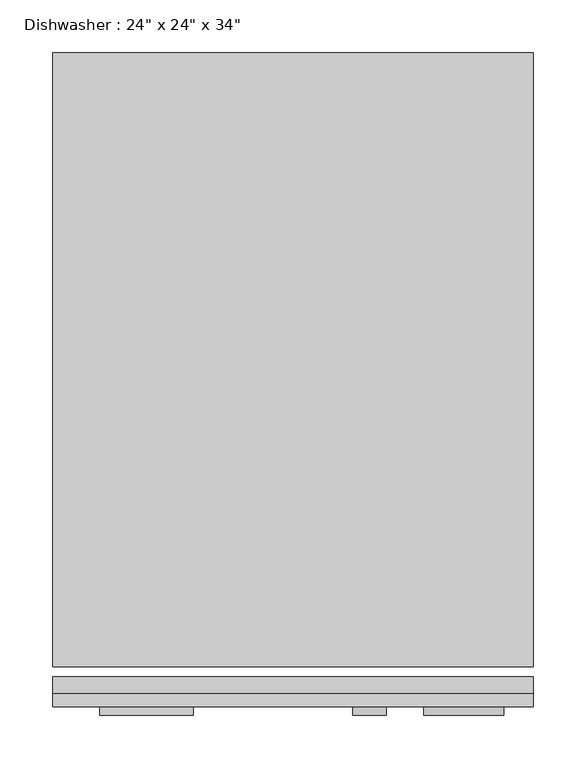
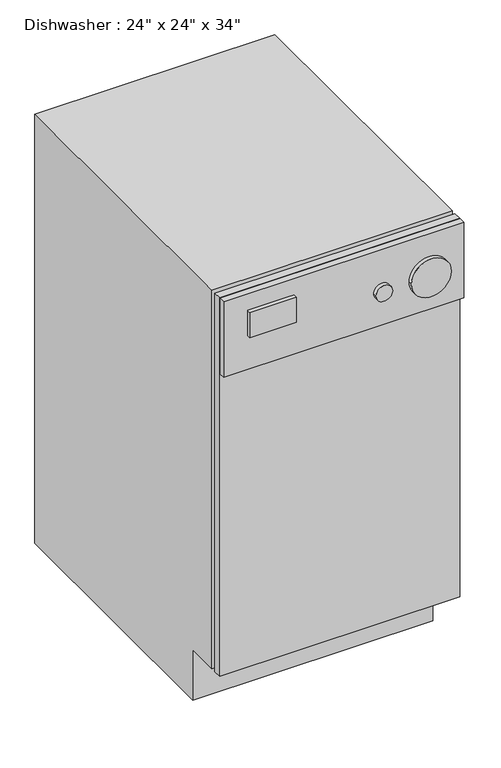
"""IFC4 building model written with IfcOpenShell, lengths in millimetres: proxy geometry."""

from ifc_helpers import new_model, si_unit, point, frame, frame_2d, origin, place, context, project, spatial, polyline, circle_curve, trimmed, segment, composite_curve, outline, extrude, source, transform, mapped, element, save


def proxy_434a9211(model_context):
    return source(origin(), model_context, "Body", "SweptSolid", [
        extrude(outline(polyline([(534.7174685, -38.3504352), (77.5174685, -38.3504352), (77.5174685, -22.4754352), (534.7174685, -22.4754352), (534.7174685, -38.3504352)])), frame((0.0, 0.0, 101.6), z_axis=(0.0, 0.0, 1.0), x_axis=(1.0, 0.0, 0.0)), (0.0, 0.0, 1.0), 762.0),
        extrude(outline(polyline([(534.7174685, -38.3504352), (534.7174685, -51.0504352), (77.5174685, -51.0504352), (77.5174685, -38.3504352), (534.7174685, -38.3504352)])), frame((0.0, 0.0, 711.2), z_axis=(0.0, 0.0, 1.0), x_axis=(1.0, 0.0, 0.0)), (0.0, 0.0, 1.0), 152.4),
        extrude(outline(polyline([(571.2495648, 0.0), (50.5495648, 0.0), (50.5495648, 101.6), (-12.9504352, 101.6), (-12.9504352, 863.6), (571.2495648, 863.6), (571.2495648, 0.0)])), frame((77.5174685, 0.0, 0.0), z_axis=(1.0, 0.0, 0.0), x_axis=(0.0, 1.0, 0.0)), (0.0, 0.0, 1.0), 457.2),
        extrude(outline(polyline([(211.4378068, -59.1863727), (122.5378068, -59.1863727), (122.5378068, -51.0504352), (211.4378068, -51.0504352), (211.4378068, -59.1863727)])), frame((0.0, 0.0, 780.0846419), z_axis=(0.0, 0.0, 1.0), x_axis=(1.0, 0.0, 0.0)), (0.0, 0.0, 1.0), 50.8),
        extrude(outline(composite_curve([segment(trimmed(circle_curve(frame_2d((780.0846419, 468.5247133)), 38.1), [point((780.0846419, 430.4247133))], [point((780.0846419, 506.6247133))], False, "CARTESIAN"), True, "CONTINUOUS"), segment(trimmed(circle_curve(frame_2d((780.0846419, 468.5247133)), 38.1), [point((780.0846419, 506.6247133))], [point((780.0846419, 430.4247133))], False, "CARTESIAN"), True, "CONTINUOUS")], self_intersect=False)), frame((0.0, -59.1863727, 0.0), z_axis=(0.0, 1.0, 0.0), x_axis=(0.0, 0.0, 1.0)), (0.0, 0.0, 1.0), 8.1359375),
        extrude(outline(composite_curve([segment(trimmed(circle_curve(frame_2d((780.0846419, 378.995318)), 15.875), [point((780.0846419, 363.120318))], [point((780.0846419, 394.870318))], False, "CARTESIAN"), True, "CONTINUOUS"), segment(trimmed(circle_curve(frame_2d((780.0846419, 378.995318)), 15.875), [point((780.0846419, 394.870318))], [point((780.0846419, 363.120318))], False, "CARTESIAN"), True, "CONTINUOUS")], self_intersect=False)), frame((0.0, -59.1863727, 0.0), z_axis=(0.0, 1.0, 0.0), x_axis=(0.0, 0.0, 1.0)), (0.0, 0.0, 1.0), 8.1359375),
    ])


if __name__ == "__main__":
    model = new_model("IFC4")
    model_context = context("Model", 3, world=origin())
    ifc_project = project(units=[si_unit("LENGTHUNIT", "METRE", prefix="MILLI")], contexts=[model_context])
    site = spatial("IfcSite", under=ifc_project)
    building = spatial("IfcBuilding", under=site)
    placement = place(None, origin())
    proxy_shape = proxy_434a9211(model_context)
    element("IfcBuildingElementProxy", 1, Name="Dishwasher : 24\" x 24\" x 34\"", ObjectType="Dishwasher : 24\" x 24\" x 34\"", at=placement, inside=building, context=model_context, shape_type="MappedRepresentation", body=[
        mapped(proxy_shape, transform((0.0, 0.0, 0.0), x_axis=(1.0, 0.0, 0.0), y_axis=(0.0, 1.0, 0.0), z_axis=(0.0, 0.0, 1.0))),
    ])
    save(model, "model.ifc")

# Revit data of these elements
# Type "Dishwasher : 24\" x 24\" x 34\""
#   Label = "DW"
#   Assembly Code = "E1090400"
#   Depth = 2' - 0"
#   Height = 2' - 10"
#   Width = 1' - 6"
#   Dishwasher Material = Steel, Paint Finish, Ivory, Glossy
#   Panel Face Material = Plastic, Opaque Black
#   Default Elevation = 0
# Element 1 (IfcBuildingElementProxy, "Dishwasher : 24\" x 24\" x 34\"")
#   Materials on its faces: "Steel, Paint Finish, Ivory, Glossy", "Plastic, Opaque Black"
# Materials
#   "Steel, Paint Finish, Ivory, Glossy": class "Metal", colour RGB 247 247 239, transparency 0, Description = "Steel, paint finish, ivory, glossy", Cost = 0
#   "Plastic, Opaque Black": class "Plastic", colour RGB 0 0 0, transparency 0.7, Description = "Plastic, generic, opaque black", Cost = 0
